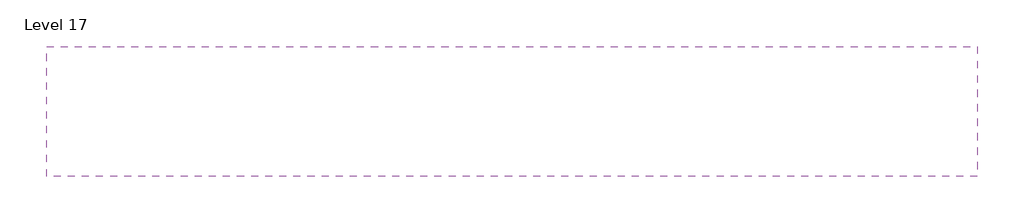
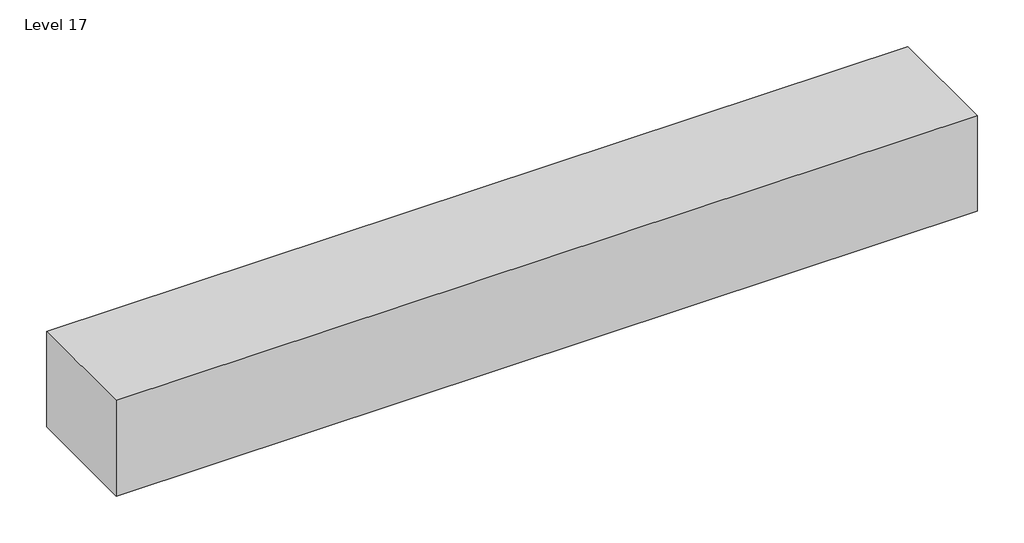
# One storey: 1 proxy.
"""IFC4 building model written with IfcOpenShell, lengths in millimetres."""

from ifc_helpers import new_model, si_unit, origin, place, context, project, spatial, transform, mapped, element, save
from components import generic_models_16_generic_models_16_89dc7be6

model = new_model("IFC4")

# Units and contexts
model_context = context("Model", 3, world=origin())
ifc_project = project(units=[si_unit("LENGTHUNIT", "METRE", prefix="MILLI")], contexts=[model_context])

# Site, building, storey
site = spatial("IfcSite", under=ifc_project)
building = spatial("IfcBuilding", under=site)
storey = spatial("IfcBuildingStorey", under=building, Name="Level 17", Elevation=26212.8)

# Proxy
placement = place(None, origin())
generic_models_16_generic_models_16_shape = generic_models_16_generic_models_16_89dc7be6(model_context)
element("IfcBuildingElementProxy", 1, Name="Generic Models 16 : Generic Models 16", ObjectType="Generic Models 16 : Generic Models 16", at=placement, inside=storey, context=model_context, shape_type="MappedRepresentation", body=[
    mapped(generic_models_16_generic_models_16_shape, transform((0.0, 0.0, 0.0), x_axis=(1.0, 0.0, 0.0), y_axis=(0.0, 1.0, 0.0), z_axis=(0.0, 0.0, 1.0))),
])

save(model, "model.ifc")

# Revit data of these elements
# Element 1 (IfcBuildingElementProxy, "Generic Models 16 : Generic Models 16")
#   Phase Created = New Construction
